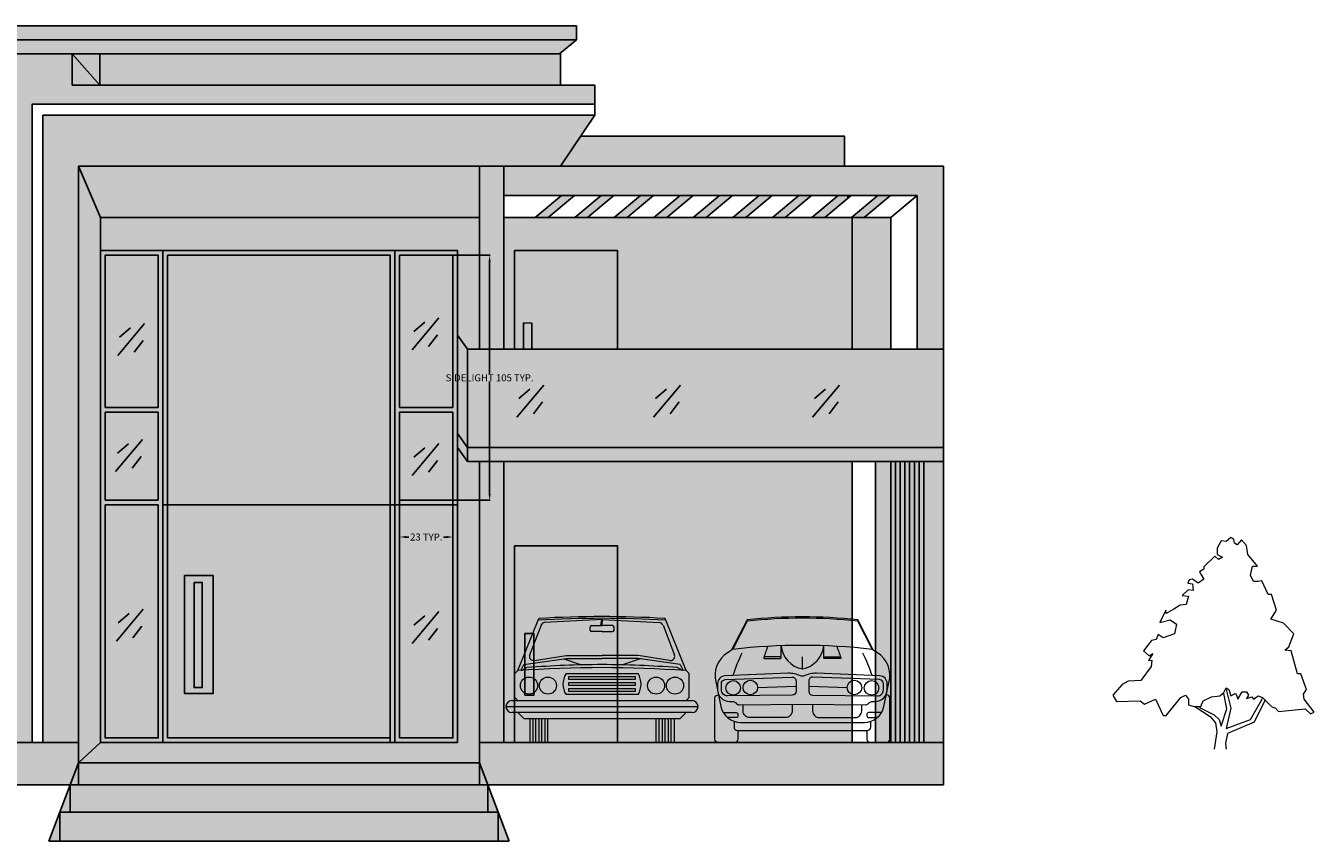
# Model space of a CAD drawing. Units: inches. Extents: x 13 to 1693, y -7 to 1519.
# Tile 7 of 10: x 292 to 842, y 1171 to 1519. Entities that reach past the tile are written whole.
import ezdxf

# ---------------------------------------------------------------- set-up
doc = ezdxf.new("R2010")
doc.units = ezdxf.units.IN
doc.header["$MEASUREMENT"] = 0
for name, color, linetype, lineweight in [('A-ANNO-DIMS', 2, 'Continuous', 18), ('A-ELEV', 7, 'Continuous', 25), ('A-ELEV-PATT', 8, 'Continuous', 13), ('A-EQPM', 8, 'Continuous', 18), ('TREE', 102, 'Continuous', 18)]:
    doc.layers.add(name, color=color, linetype=linetype, lineweight=lineweight)
doc.styles.get("Standard").update_dxf_attribs({"font": 'arial.ttf'})
doc.dimstyles.get("Standard").update_dxf_attribs({"dimtxt": 3, "dimasz": 2.68, "dimexe": 0.18, "dimexo": 0.0625, "dimgap": 0.09, "dimtad": 0, "dimtih": 1, "dimtoh": 1, "dimdec": 0, "dimzin": 0, "dimdsep": 46, "dimlunit": 3, "dimtxsty": 'Standard', "dimcen": 0.09, "dimadec": 0, "dimazin": 0, "dimtfac": 1, "dimtdec": 0, "dimtofl": 0, "dimtmove": 0, "dimatfit": 3, "dimfxl": 1, "dimtolj": 1, "dimtzin": 0, "dimarcsym": 0})

# ---------------------------------------------------------------- blocks, each defined once
blk = doc.blocks.new('*U27')
for p, q in [((-37.38, 32.04), (-28.11, 55.23)), ((-0.21, 54.74), (-0.67, 52.07)), ((0.21, 54.74), (-0.23, 52.08)), ((37.38, 32.04), (28.11, 55.23)), ((-36.05, 32.04), (-34.71, 34.71)), ((-34.71, 34.71), (-16.02, 37.38)), ((-16.94, 37.24), (-9.08, 34.62)), ((-16.02, 37.38), (0, 37.38)), ((16.02, 37.38), (0, 37.38)), ((16.93, 37.24), (9.08, 34.62)), ((34.71, 34.71), (16.02, 37.38)), ((34.71, 34.71), (36.05, 32.04)), ((-38.72, 30.71), (-37.38, 32.04)), ((-38.72, 20.03), (-38.72, 30.71)), ((-35.8, 32.16), (-33.38, 33.38)), ((-16.02, 30.71), (16.02, 30.71)), ((-14.69, 29.37), (14.69, 29.37)), ((-14.69, 28.04), (-14.69, 29.37)), ((14.69, 29.37), (14.69, 28.04)), ((35.8, 32.16), (33.38, 33.38)), ((38.72, 30.71), (37.38, 32.04)), ((38.72, 20.03), (38.72, 30.71)), ((14.69, 28.04), (-14.69, 28.04)), ((-14.69, 26.7), (14.69, 26.7)), ((-14.69, 25.37), (-14.69, 26.7)), ((14.69, 25.37), (-14.69, 25.37)), ((-14.69, 24.03), (14.69, 24.03)), ((-14.69, 22.7), (-14.69, 24.03)), ((14.69, 26.7), (14.69, 25.37)), ((14.69, 24.03), (14.69, 22.7)), ((-40.05, 18.69), (40.05, 18.69)), ((-37.38, 18.69), (-38.72, 20.03)), ((16.02, 21.36), (-16.02, 21.36)), ((14.69, 22.7), (-14.69, 22.7)), ((37.38, 18.69), (38.72, 20.03)), ((-42.72, 16.02), (42.72, 16.02)), ((40.05, 13.35), (-40.05, 13.35)), ((-37.38, 13.35), (-34.71, 10.68)), ((34.71, 10.68), (37.38, 13.35)), ((-34.71, 10.68), (34.71, 10.68)), ((-32.04, 10.68), (-32.04, 0)), ((-30.71, 10.68), (-30.71, 0)), ((-29.37, 0), (-29.37, 10.68)), ((-28.04, 10.68), (-28.04, 0)), ((-26.7, 0), (-26.7, 10.68)), ((-25.37, 10.68), (-25.37, 0)), ((-24.03, 0), (-24.03, 10.68)), ((24.03, 0), (24.03, 10.68)), ((25.37, 0), (25.37, 10.68)), ((26.7, 10.68), (26.7, 0)), ((28.04, 0), (28.04, 10.68)), ((29.37, 10.68), (29.37, 0)), ((30.71, 0), (30.71, 10.68)), ((32.04, 10.68), (32.04, 0)), ((-32.04, 0), (-24.03, 0)), ((32.04, 0), (24.03, 0))]:
    blk.add_line(p, q)
for points in [[(-27.12, 52.31), (-32.28, 38.89)], [(0, 54.74), (-25.63, 53.46)], [(-4.67, 52.07), (0, 52.07)], [(4.67, 52.07), (0, 52.07)], [(0.01, 54.74), (25.64, 53.45)], [(27.13, 52.3), (32.28, 38.88)], [(-5.34, 50.07), (-5.34, 51.4)], [(0, 49.4), (-4.67, 49.4)], [(0, 49.4), (4.67, 49.4)], [(5.34, 50.07), (5.34, 51.4)], [(-30.06, 36.56), (-16.02, 38.72), (0, 38.72)], [(30.06, 36.54), (16.02, 38.71), (0, 38.72)]]:
    blk.add_lwpolyline(points)
for centre in [(-32.47, 25.37), (-24.06, 25.37), (24.06, 25.37), (32.47, 25.37)]:
    blk.add_circle(centre, 3.8)
for centre, radius, start, end in [((0, -432), 487.32, 86.65721, 93.3419), ((0, -431.24), 487.32, 86.69396, 93.3033), ((-25.37, 51.59), 1.89, 97.4497, 154.9311), ((-4.67, 51.4), 0.668, 93.60832, 178.1081), ((4.67, 51.4), 0.668, 1.89193, 86.39168), ((25.37, 51.57), 1.89, 25.04208, 82.52346), ((-4.67, 50.07), 0.668, 184.4192, 266.4386), ((4.67, 50.07), 0.668, 273.5614, 355.5808), ((0.67, -399.87), 434.58, 90.08801, 94.49321), ((-30.43, 38.42), 1.89, 166.5724, 279.9572), ((-0.67, -399.87), 434.58, 85.50679, 89.91199), ((30.43, 38.41), 1.89, 260.016, 13.40079), ((0, -490.66), 524.03, 85.90918, 94.09081), ((-8.68, 26.03), 8.7, 147.5288, 212.4712), ((8.68, 26.03), 8.7, 327.5288, 32.47119), ((-40.05, 16.02), 2.67, 90, 270), ((40.05, 16.02), 2.67, 270, 90)]:
    blk.add_arc(centre, radius, start, end)
blk = doc.blocks.new('*U28')
for p, q in [((-9.51, 37.84), (-9.51, 43.25)), ((9.51, 37.84), (9.51, 43.25)), ((0, 32.82), (0, 38.19)), ((-19.91, 24.53), (-2.81, 25.14)), ((2.81, 25.14), (19.91, 24.53))]:
    blk.add_line(p, q)
for points in [[(-38.83, 28.63), (-36.22, 16.07, 0.355359), (-27.52, 9), (27.58, 9, 0.355331), (36.28, 16.07), (38.89, 28.63, 0.324597), (31.68, 40.93), (24.69, 54.68, 0.052145), (-24.63, 54.68), (-31.63, 40.93, 0.324597)], [(-24.58, 54.09), (-30.92, 41.61), (-30.92, 41.61, -0.059427), (30.98, 41.61), (24.64, 54.09, 0.05217)], [(-16.8, 37.38), (-9.88, 37.38, 0.414214), (-9.51, 37.75), (-9.51, 37.82, 0.414214), (-9.88, 38.19), (-16.8, 38.19, 0.414214), (-17.17, 37.82), (-17.17, 37.75, 0.414214)], [(16.8, 37.38), (9.88, 37.38, -0.414214), (9.51, 37.75), (9.51, 37.82, -0.414214), (9.88, 38.19), (16.8, 38.19, -0.414214), (17.17, 37.82), (17.17, 37.75, -0.414214)], [(-4.66, 29.17, -0.427329), (-2.81, 27.41), (-2.81, 22.88, -0.410558), (-4.56, 21.11), (-33.36, 20.8, -0.417878), (-36.04, 23.45), (-36.04, 26.26, -0.401219), (-34.35, 28.03)], [(4.66, 29.17, 0.427329), (2.81, 27.41), (2.81, 22.88, 0.410558), (4.56, 21.11), (33.36, 20.8, 0.417878), (36.04, 23.45), (36.04, 26.26, 0.401219), (34.35, 28.03)]]:
    blk.add_lwpolyline(points, format="xyb", close=True)
for points in [[(-6.29, 30.92), (-34.43, 29.71, 0.401219), (-37.73, 26.26), (-37.73, 23.63, 0.414214), (-32.43, 18.34), (-31.07, 18.34, -0.198912), (-29.82, 17.82), (-29.29, 17.29, 0.202778), (-28.01, 16.77), (0, 17.13), (28.01, 16.77, 0.202778), (29.29, 17.29), (29.82, 17.82, -0.198912), (31.07, 18.34), (32.43, 18.34, 0.414214), (37.73, 23.63), (37.73, 26.26, 0.401219), (34.43, 29.71), (6.29, 30.92)], [(6.29, 30.92, 0.105807), (0.87, 29.72, -0.131652), (-0.87, 29.72, 0.105807), (-6.29, 30.92)], [(-28.7, 5.37), (-28.7, 1.48, -0.414214), (-30.18, 0), (-37.41, 0, -0.414214), (-38.89, 1.48), (-38.89, 19.74, -0.414214), (-37.41, 21.22), (-37.29, 21.22)], [(28.7, 5.37), (28.7, 1.48, 0.414214), (30.18, 0), (37.41, 0, 0.414214), (38.89, 1.48), (38.89, 19.74, 0.414214), (37.41, 21.22), (37.35, 21.22)], [(-35.17, 13.37), (-29.44, 13.37, -0.414214), (-28.7, 12.63), (-28.7, 11.88, -0.414214), (-29.44, 11.14), (-33.31, 11.14)], [(-4.56, 17.07), (-4.56, 14.1, -0.414214), (-7.52, 11.14), (-23.43, 11.14, -0.414214), (-26.39, 14.1), (-26.39, 16.79)], [(4.56, 17.07), (4.56, 14.1, 0.414214), (7.52, 11.14), (23.43, 11.14, 0.414214), (26.39, 14.1), (26.39, 16.79)], [(35.17, 13.37), (29.44, 13.37, 0.414214), (28.7, 12.63), (28.7, 11.88, 0.414214), (29.44, 11.14), (33.31, 11.14)], [(-30.39, 9.47), (-30.39, 6.85, 0.414214), (-28.91, 5.37), (28.91, 5.37, 0.414214), (30.39, 6.85), (30.39, 9.47)]]:
    blk.add_lwpolyline(points, format="xyb")
for centre in [(-30.79, 24.36), (-23.15, 24.53), (23.15, 24.53), (30.79, 24.36)]:
    blk.add_circle(centre, 3.24)
for centre, radius, start, end in [((41.5, 19.77), 61.38, 157.83365, 162.90143), ((2.03, 44.22), 11.58, 184.78179, 259.90449), ((-2.03, 44.22), 11.58, 280.09551, 355.21821), ((-41.5, 19.77), 61.38, 17.09857, 22.16635), ((27.74, 11.77), 61.38, 152.82966, 162.90143), ((-27.69, 11.77), 61.38, 17.09857, 27.17034)]:
    blk.add_arc(centre, radius, start, end)
blk = doc.blocks.new('*U31')
for points in [[(22.0124, 137.721), (18.5475, 141.5624), (15.5282, 138.2446), (13.8028, 139.3505), (13.3714, 142.1153), (11.2148, 143.2214), (8.1954, 140.4564), (4.7447, 141.0094), (2.1567, 136.0326), (2.1567, 131.6088), (5.6074, 129.9499), (3.0193, 128.2909), (0.4313, 130.5029), (-6.9015, 123.3141), (-6.9015, 121.6552), (-9.9208, 119.9963), (-9.0581, 118.3373), (-6.9015, 115.0195), (-10.7835, 112.2546), (-14.6656, 115.0195), (-16.8222, 114.4665), (-17.6849, 112.2546), (-14.6656, 111.7016), (-14.2342, 107.2778), (-17.6065, 107.8307), (-21.5669, 103.9599), (-17.2536, 103.4069), (-18.9789, 97.8771), (-22.8609, 97.3241), (-27.1743, 94.5593), (-32.3504, 91.7944), (-32.7817, 94.0063), (-36.6638, 85.7116), (-29.7624, 87.3705), (-25.449, 84.6056), (-26.743, 77.9699), (-34.507, 75.205), (-37.9578, 77.4169), (-39.2518, 74.099), (-42.2711, 73.5461), (-44.8592, 70.2282), (-47.8786, 66.3574), (-43.9965, 63.0395), (-41.4085, 64.6985), (-44.3346, 59.8898), (-42.2089, 60.1377), (-42.5159, 55.7849), (-49.6039, 46.4502), (-58.2307, 45.8972), (-62.1127, 43.6853), (-68.5828, 36.4966), (-65.9947, 32.0727), (-50.0352, 32.6257), (-47.0159, 30.4138), (-39.6831, 33.7317), (-34.507, 22.6721), (-32.3504, 22.6721), (-22.4296, 34.8376), (-19.4102, 36.4966), (-17.2536, 33.7317), (-17.2536, 29.8608), (-13.8028, 28.7549), (-9.0581, 28.7549), (-7.3328, 32.6257), (-1.7254, 35.3906), (3.8821, 35.9436), (6.4701, 38.1555), (6.9014, 38.7085), (8.1954, 41.4734), (9.9208, 40.3674), (11.2148, 35.9436), (14.2341, 37.6025), (15.0968, 36.4966), (15.9595, 33.7317), (18.9789, 38.7085), (21.9982, 38.7085), (23.2922, 36.4966), (21.9982, 34.2847), (25.4489, 35.3906), (26.743, 33.7317), (29.7623, 35.9436), (32.7817, 34.8376), (38.8204, 28.7549), (41.4084, 27.6489), (43.5651, 25.437), (61.6813, 27.0959), (65.132, 23.7781), (67.7201, 24.884), (60.8186, 33.7317), (60.3873, 37.0495), (62.544, 40.3674), (58.662, 50.874), (56.5053, 50.874), (52.1919, 66.3574), (47.8785, 66.9103), (50.4665, 69.1222), (53.9172, 77.9699), (47.0158, 85.1586), (38.3891, 87.9235), (42.2711, 94.0063)], [(42.2711, 94.0063), (38.8204, 104.5129), (36.6637, 104.5129), (32.3503, 113.9135), (29.7623, 113.3605), (26.743, 113.3605), (24.5862, 117.7844), (25.8802, 123.8671), (29.331, 123.8671), (22.8609, 131.6088), (21.9982, 137.6916)], [(-9.9208, 28.2019), (0, 23.2251), (3.4507, 19.9072), (4.7447, 15.4834), (8.6267, 27.0959), (6.4701, 37.6025)], [(8.1954, 40.3674), (11.2148, 27.6489), (8.1954, 13.8245), (24.5862, 19.9072), (32.7817, 34.2847)], [(-12.9401, 28.7549), (-2.588, 22.1191), (0.8626, 17.6953), (1.7253, 11.6125), (0, 0)], [(34.5071, 33.1787), (27.1743, 18.2483), (9.0581, 10.5066), (7.7641, 3.8708), (8.1954, 0)]]:
    blk.add_lwpolyline(points)
blk = doc.blocks.new('ELEV-SIDELIGHT')
for p, q in [((22.68, 39.67), (0, 39.67)), ((22.68, 37.67), (0, 37.67)), ((0, 0), (22.68, 0))]:
    blk.add_line(p, q)
for points in [[(0, 39.67), (0, 104.56), (22.68, 104.56), (22.68, 39.67)], [(0, 0), (0, 37.67)], [(22.68, 37.67), (22.68, 0)]]:
    blk.add_lwpolyline(points)
blk = doc.blocks.new('*D66')
at = {"layer": 'A-ANNO-DIMS', "color": 0, "lineweight": -2, "transparency": 16777216}
for p, q in [((474.2, 1421.23), (490, 1421.23)), ((489.82, 1418.55), (489.82, 1370.59)), ((489.82, 1319.35), (489.82, 1367.31)), ((474.2, 1316.67), (490, 1316.67))]:
    blk.add_line(p, q, dxfattribs=at)
at = {"layer": 'A-ANNO-DIMS', "color": 0, "transparency": 16777216}
for points in [[(489.37, 1418.55), (490.27, 1418.55), (489.82, 1421.23)], [(489.37, 1319.35), (490.27, 1319.35), (489.82, 1316.67)]]:
    blk.add_solid(points, dxfattribs=at)
at = {"layer": 'Defpoints', "color": 0, "transparency": 16777216}
for p in [(474.14, 1421.23), (489.82, 1421.23), (474.14, 1316.67)]:
    blk.add_point(p, dxfattribs=at)
at = {"layer": 'A-ANNO-DIMS', "color": 0, "transparency": 16777216, "insert": (489.82, 1368.95), "char_height": 3, "attachment_point": 5}
blk.add_mtext('\\A1;SIDELIGHT 105 TYP.', dxfattribs=at)
blk = doc.blocks.new('*D67')
at = {"layer": 'A-ANNO-DIMS', "color": 0, "lineweight": -2, "transparency": 16777216}
for p, q in [((451.45, 1316.61), (451.45, 1300.81)), ((474.14, 1316.61), (474.14, 1300.81)), ((454.13, 1300.99), (455.38, 1300.99)), ((471.46, 1300.99), (470.21, 1300.99))]:
    blk.add_line(p, q, dxfattribs=at)
at = {"layer": 'A-ANNO-DIMS', "color": 0, "transparency": 16777216}
for points in [[(454.13, 1301.43), (454.13, 1300.54), (451.45, 1300.99)], [(471.46, 1301.43), (471.46, 1300.54), (474.14, 1300.99)]]:
    blk.add_solid(points, dxfattribs=at)
at = {"layer": 'Defpoints', "color": 0, "transparency": 16777216}
for p in [(451.45, 1316.67), (474.14, 1316.67), (474.14, 1300.99)]:
    blk.add_point(p, dxfattribs=at)
at = {"layer": 'A-ANNO-DIMS', "color": 0, "transparency": 16777216, "insert": (462.8, 1300.99), "char_height": 3, "attachment_point": 5}
blk.add_mtext('\\A1;23 TYP.', dxfattribs=at)

msp = doc.modelspace()

# ---------------------------------------------------------------- hatches: boundary and pattern name
at = {"layer": 'A-ELEV-PATT'}
h = msp.add_hatch(color=256, dxfattribs=at)
h.dxf.hatch_style = 1
h.paths.add_polyline_path([(526.9, 1519.22), (247.4, 1519.22), (247.4, 1513.22), (526.9, 1513.22)])
h = msp.add_hatch(color=256, dxfattribs=at)
h.dxf.hatch_style = 1
h.paths.add_polyline_path([(485.45, 1459.23), (314.45, 1459.23), (323.77, 1437.38), (485.45, 1437.38)])
h.paths.add_polyline_path([(323.77, 1437.38), (314.45, 1459.23), (314.45, 1204.63), (323.77, 1213.23), (323.77, 1423.23)])
h.paths.add_polyline_path([(526.9, 1513.22), (247.4, 1513.22), (267.64, 1507.23), (519.7, 1507.23)])
h = msp.add_hatch(color=256, dxfattribs=at)
h.dxf.hatch_style = 1
h.paths.add_polyline_path([(534.67, 1493.81), (311.73, 1493.81), (311.73, 1507.23), (169.4, 1507.23), (169.4, 1457.61), (259.19, 1457.61), (259.19, 1213.23), (294.63, 1213.23), (294.63, 1485.7), (299.21, 1485.7), (534.67, 1485.7)])
h.paths.add_polyline_path([(534.67, 1481.12), (299.21, 1481.12), (299.21, 1213.23), (314.45, 1213.23), (314.45, 1459.23), (520.13, 1459.23)], flags=17)
h.paths.add_polyline_path([(146.87, 1507.23), (116.45, 1507.23), (116.45, 1339.23), (116.45, 1213.23), (129.66, 1213.23), (129.66, 1457.61), (146.87, 1457.61)])
h.paths.add_polyline_path([(151, 1507.23), (148.74, 1507.23), (148.74, 1457.61), (151, 1457.61)])
h.paths.add_polyline_path([(155.13, 1507.23), (152.87, 1507.23), (152.87, 1457.61), (155.13, 1457.61)])
h.paths.add_polyline_path([(159.26, 1507.23), (157.01, 1507.23), (157.01, 1457.61), (159.26, 1457.61)])
h.paths.add_polyline_path([(163.39, 1507.23), (161.14, 1507.23), (161.14, 1457.61), (163.39, 1457.61)])
h.paths.add_polyline_path([(167.53, 1507.23), (165.27, 1507.23), (165.27, 1457.61), (167.53, 1457.61)])
h = msp.add_hatch(color=256, dxfattribs=at)
h.dxf.hatch_style = 1
h.paths.add_polyline_path([(323.53, 1507.23), (311.73, 1507.23), (323.53, 1493.81)], flags=17)
h.paths.add_polyline_path([(311.73, 1507.23), (311.73, 1493.81), (323.53, 1493.81)])
h = msp.add_hatch(color=256, dxfattribs=at)
h.dxf.hatch_style = 1
h.paths.add_polyline_path([(520.13, 1507.59), (519.7, 1507.23), (323.53, 1507.23), (323.53, 1493.81), (520.13, 1493.81)])
h = msp.add_hatch(color=256, dxfattribs=at)
h.dxf.hatch_style = 1
h.paths.add_polyline_path([(641.26, 1472.05), (528.65, 1472.05), (520.13, 1459.23), (641.26, 1459.23)])
h = msp.add_hatch(color=256, dxfattribs=at)
h.dxf.hatch_style = 1
h.paths.add_polyline_path([(495.89, 1459.23), (485.45, 1459.23), (485.45, 1381.23), (495.89, 1381.23)])
h.paths.add_polyline_path([(495.89, 1333.23), (485.45, 1333.23), (485.45, 1213.23), (495.89, 1213.23)])
h = msp.add_hatch(color=256, dxfattribs=at)
h.dxf.hatch_style = 1
h.paths.add_polyline_path([(683.45, 1459.23), (495.89, 1459.23), (495.89, 1446.73), (672.26, 1446.73), (672.26, 1381.23), (683.45, 1381.23)])
h.paths.add_polyline_path([(661.02, 1437.38), (644.49, 1437.38), (644.49, 1381.23), (661.02, 1381.23)], flags=17)
h = msp.add_hatch(color=256, dxfattribs=at)
h.dxf.hatch_style = 1
h.paths.add_polyline_path([(526.03, 1446.73), (520.54, 1446.73), (509.3, 1437.38), (514.79, 1437.38)])
h.paths.add_polyline_path([(542.89, 1446.73), (537.4, 1446.73), (526.16, 1437.38), (531.65, 1437.38)])
h.paths.add_polyline_path([(559.75, 1446.73), (554.25, 1446.73), (543.02, 1437.38), (548.51, 1437.38)])
h.paths.add_polyline_path([(576.6, 1446.73), (571.11, 1446.73), (559.87, 1437.38), (565.37, 1437.38)])
h.paths.add_polyline_path([(593.46, 1446.73), (587.97, 1446.73), (576.73, 1437.38), (582.22, 1437.38)])
h.paths.add_polyline_path([(610.32, 1446.73), (604.83, 1446.73), (593.59, 1437.38), (599.08, 1437.38)])
h.paths.add_polyline_path([(627.18, 1446.73), (621.68, 1446.73), (610.45, 1437.38), (615.94, 1437.38)])
h.paths.add_polyline_path([(642.63, 1445.56), (642.63, 1446.73), (638.54, 1446.73), (627.3, 1437.38), (632.8, 1437.38)])
h.paths.add_polyline_path([(660.89, 1446.73), (655.4, 1446.73), (644.16, 1437.38), (649.65, 1437.38)])
h = msp.add_hatch(color=256, dxfattribs=at)
h.dxf.hatch_style = 1
h.paths.add_polyline_path([(644.49, 1333.23), (495.89, 1333.23), (495.89, 1213.23), (500.45, 1213.23), (500.45, 1297.23), (544.41, 1297.23), (544.41, 1213.23), (644.49, 1213.23)])
h.paths.add_polyline_path([(644.49, 1437.38), (495.89, 1437.38), (495.89, 1381.23), (500.45, 1381.23), (500.45, 1423.23), (544.41, 1423.23), (544.41, 1381.23), (644.49, 1381.23)])
h.paths.add_polyline_path([(485.45, 1437.38), (323.77, 1437.38), (323.77, 1423.23), (350.45, 1423.23), (449.45, 1423.23), (476.14, 1423.23), (476.14, 1387.14), (480.46, 1381.23), (485.45, 1381.23)])
h.paths.add_polyline_path([(485.45, 1333.23), (480.46, 1333.23), (476.14, 1339.14), (476.14, 1213.23), (449.45, 1213.23), (323.77, 1213.23), (314.45, 1204.63), (485.45, 1204.63)])
at = {"layer": 'A-ELEV-PATT', "transparency": 33554592}
h = msp.add_hatch(color=256, dxfattribs=at)
h.dxf.hatch_style = 1
h.paths.add_polyline_path([(202.48, 1421.23), (175.34, 1421.23), (175.34, 1381.23), (175.34, 1354.34), (202.48, 1354.34)])
h.paths.add_polyline_path([(226.48, 1421.23), (211.36, 1421.23), (204.48, 1421.23), (204.48, 1354.34), (226.48, 1354.34)])
h.paths.add_polyline_path([(259.19, 1421.23), (228.48, 1421.23), (228.48, 1354.34), (259.19, 1354.34)])
h.paths.add_polyline_path([(259.19, 1316.67), (230.48, 1316.67), (230.48, 1251.23), (259.19, 1251.23)])
h.paths.add_polyline_path([(228.48, 1316.67), (206.48, 1316.67), (206.48, 1251.23), (228.48, 1251.23)])
h.paths.add_polyline_path([(204.48, 1316.67), (175.34, 1316.67), (175.34, 1297.23), (175.34, 1251.23), (204.48, 1251.23)])
h.paths.add_polyline_path([(480.46, 1381.23), (476.14, 1387.14), (476.14, 1345.14), (480.46, 1339.23)])
h.paths.add_polyline_path([(683.45, 1381.23), (480.46, 1381.23), (480.46, 1339.23), (683.45, 1339.23)])
h.paths.add_polyline_path([(348.45, 1421.23), (325.77, 1421.23), (325.77, 1356.34), (348.45, 1356.34)])
h.paths.add_polyline_path([(474.14, 1421.23), (451.45, 1421.23), (451.45, 1356.34), (474.14, 1356.34)])
h.paths.add_polyline_path([(474.14, 1354.34), (451.45, 1354.34), (451.45, 1316.67), (474.14, 1316.67)])
h.paths.add_polyline_path([(348.45, 1354.34), (325.77, 1354.34), (325.77, 1316.67), (348.45, 1316.67)])
h.paths.add_polyline_path([(348.45, 1314.67), (325.77, 1314.67), (325.77, 1215.23), (348.45, 1215.23)])
h.paths.add_polyline_path([(474.14, 1314.67), (451.45, 1314.67), (451.45, 1215.23), (474.14, 1215.23)])
at = {"layer": 'A-ELEV-PATT'}
h = msp.add_hatch(color=256, dxfattribs=at)
h.dxf.hatch_style = 1
h.paths.add_polyline_path([(350.45, 1423.23), (323.77, 1423.23), (323.77, 1213.23), (350.45, 1213.23)])
h.paths.add_polyline_path([(325.77, 1356.34), (325.77, 1421.23), (348.45, 1421.23), (348.45, 1356.34)], flags=16)
h.paths.add_polyline_path([(348.45, 1354.34), (348.45, 1316.67), (325.77, 1316.67), (325.77, 1354.34)], flags=16)
h.paths.add_polyline_path([(348.45, 1314.67), (348.45, 1215.23), (325.77, 1215.23), (325.77, 1314.67)], flags=16)
h = msp.add_hatch(color=256, dxfattribs=at)
h.dxf.hatch_style = 1
h.paths.add_polyline_path([(449.45, 1423.23), (350.45, 1423.23), (350.45, 1375.23), (350.45, 1314.67), (352.45, 1314.67), (352.45, 1375.23), (352.45, 1421.23), (447.45, 1421.23), (447.45, 1375.23), (447.45, 1314.67), (449.45, 1314.67), (449.45, 1375.23)])
h = msp.add_hatch(color=256, dxfattribs=at)
h.dxf.hatch_style = 1
h.paths.add_polyline_path([(447.45, 1375.23), (447.45, 1421.23), (352.45, 1421.23), (352.45, 1375.23), (352.45, 1314.67), (447.45, 1314.67)])
h = msp.add_hatch(color=256, dxfattribs=at)
h.dxf.hatch_style = 1
h.paths.add_polyline_path([(476.14, 1423.23), (449.45, 1423.23), (449.45, 1314.67), (476.14, 1314.67)])
h.paths.add_polyline_path([(474.14, 1356.34), (451.45, 1356.34), (451.45, 1421.23), (474.14, 1421.23)], flags=16)
h.paths.add_polyline_path([(474.14, 1354.34), (474.14, 1316.67), (451.45, 1316.67), (451.45, 1354.34)], flags=16)
h.paths.add_polyline_path([(476.14, 1314.67), (474.14, 1314.67), (474.14, 1215.23), (451.45, 1215.23), (451.45, 1314.67), (449.45, 1314.67), (449.45, 1213.23), (476.14, 1213.23)])
h = msp.add_hatch(color=256, dxfattribs=at)
h.dxf.hatch_style = 1
h.paths.add_polyline_path([(544.41, 1423.23), (500.45, 1423.23), (500.45, 1381.23), (504.32, 1381.23), (504.32, 1392.37), (507.79, 1392.31), (507.79, 1381.23), (544.41, 1381.23)])
h = msp.add_hatch(color=256, dxfattribs=at)
h.dxf.hatch_style = 1
h.paths.add_polyline_path([(507.79, 1392.31), (504.32, 1392.37), (504.32, 1381.3), (507.79, 1381.23)])
h = msp.add_hatch(color=256, dxfattribs=at)
h.dxf.hatch_style = 1
h.paths.add_polyline_path([(683.45, 1339.23), (480.46, 1339.23), (480.46, 1333.23), (683.45, 1333.23)])
h.paths.add_polyline_path([(476.14, 1345.14), (476.14, 1339.14), (480.46, 1333.23), (480.46, 1339.23)])
h = msp.add_hatch(color=256, dxfattribs=at)
h.dxf.hatch_style = 1
h.paths.add_polyline_path([(661.02, 1333.23), (654.43, 1333.23), (654.43, 1213.23), (661.02, 1213.23)])
h = msp.add_hatch(color=256, dxfattribs=at)
h.dxf.hatch_style = 1
h.paths.add_polyline_path([(663.02, 1333.23), (661.02, 1333.23), (661.02, 1213.23), (663.02, 1213.23)])
h.paths.add_polyline_path([(667.02, 1333.23), (665.02, 1333.23), (665.02, 1213.23), (667.02, 1213.23)])
h.paths.add_polyline_path([(671.02, 1333.23), (669.02, 1333.23), (669.02, 1213.23), (671.02, 1213.23)])
h.paths.add_polyline_path([(665.02, 1333.23), (663.02, 1333.23), (663.02, 1213.23), (665.02, 1213.23)])
h = msp.add_hatch(color=256, dxfattribs=at)
h.dxf.hatch_style = 1
h.paths.add_polyline_path([(665.02, 1333.23), (663.02, 1333.23), (663.02, 1213.23)])
h = msp.add_hatch(color=256, dxfattribs=at)
h.dxf.hatch_style = 1
h.paths.add_polyline_path([(673.02, 1333.23), (671.02, 1333.23), (671.02, 1213.23), (673.02, 1213.23)])
h.paths.add_polyline_path([(675.02, 1333.23), (673.02, 1333.23), (673.02, 1213.23), (675.02, 1213.23)])
h.paths.add_polyline_path([(669.02, 1333.23), (667.02, 1333.23), (667.02, 1213.23), (669.02, 1213.23)])
h = msp.add_hatch(color=256, dxfattribs=at)
h.dxf.hatch_style = 1
h.paths.add_polyline_path([(683.45, 1333.23), (675.02, 1333.23), (675.02, 1213.23), (683.45, 1213.23)])
h = msp.add_hatch(color=256, dxfattribs=at)
h.dxf.hatch_style = 1
h.paths.add_polyline_path([(352.45, 1314.67), (350.45, 1314.67), (350.45, 1297.23), (350.45, 1213.23), (399.95, 1213.23), (447.45, 1213.23), (447.45, 1215.23), (399.95, 1215.23), (352.45, 1215.23), (352.45, 1297.23)])
h.paths.add_polyline_path([(449.45, 1297.23), (449.45, 1314.67), (447.45, 1314.67), (447.45, 1213.23), (449.45, 1213.23)])
h = msp.add_hatch(color=256, dxfattribs=at)
h.dxf.hatch_style = 1
h.paths.add_polyline_path([(352.45, 1314.67), (352.45, 1297.23), (352.45, 1215.23), (399.95, 1215.23), (447.45, 1215.23), (447.45, 1297.23), (447.45, 1314.67)])
h.paths.add_polyline_path([(371.9, 1284.52), (371.9, 1234.22), (359.62, 1234.22), (359.62, 1284.52)], flags=16)
h = msp.add_hatch(color=256, dxfattribs=at)
h.dxf.hatch_style = 1
h.paths.add_polyline_path([(544.41, 1297.23), (500.45, 1297.23), (500.45, 1213.23), (544.41, 1213.23)])
h.paths.add_polyline_path([(508.74, 1259.76), (508.74, 1233.51), (504.9, 1233.51), (504.9, 1259.76)], flags=16)
h = msp.add_hatch(color=256, dxfattribs=at)
h.dxf.hatch_style = 1
h.paths.add_polyline_path([(359.62, 1284.52), (359.62, 1234.22), (371.9, 1234.22), (371.9, 1284.52)])
h = msp.add_hatch(color=256, dxfattribs=at)
h.dxf.hatch_style = 1
h.paths.add_polyline_path([(367.22, 1281.62), (363.72, 1281.62), (363.72, 1236.7), (367.22, 1236.7)])
h = msp.add_hatch(color=256, dxfattribs=at)
h.dxf.hatch_style = 1
h.paths.add_polyline_path([(508.74, 1259.76), (504.9, 1259.76), (504.9, 1233.51), (508.74, 1233.51)])
h = msp.add_hatch(dxfattribs=at)
h.set_pattern_fill('AR-CONC', color=256)
h.set_pattern_definition([(50, (-1203.873, -530.7854), (7.172602, -0.627521), [0.75, -8.25]), (355, (-1203.873, -530.785), (-1.387513, 7.521921), [0.6, -6.6]), (100.45144, (-1203.2755, -530.8376), (5.785088, 6.8944), [0.637402, -7.011421]), (46.1842, (-1203.873, -528.785), (10.672413, -1.655193), [1.125, -12.375]), (96.63564, (-1202.984, -528.923), (9.34662, 9.741186), [0.956103, -10.517138]), (351.18416, (-1203.873, -528.785), (9.34662, 9.741186), [0.9, -9.9]), (21, (-1202.873, -529.2854), (5.96907, -4.026189), [0.75, -8.25]), (326, (-1202.873, -529.285), (2.433153, 7.2515), [0.6, -6.6]), (71.45144, (-1202.376, -529.621), (8.402224, 3.225312), [0.637402, -7.011421]), (37.5, (-1203.8732, -530.7854), (0.1215986, 3.3289385), [0, -6.52, 0, -6.7, 0, -6.625]), (7.5, (-1203.8732, -530.7854), (2.6306954, 3.944117), [0, -3.82, 0, -6.37, 0, -2.525]), (327.5, (-1206.1032, -530.7854), (5.3382244, -0.2255487), [0, -2.5, 0, -7.8, 0, -10.35]), (317.5, (-1207.103, -530.7854), (5.831862, 1.00105), [0, -3.25, 0, -5.18, 0, -7.35])])
h.paths.add_polyline_path([(314.45, 1213.23), (116.45, 1213.23), (116.45, 1195.23), (310.89, 1195.23), (314.45, 1204.63)])
h.paths.add_polyline_path([(683.45, 1213.23), (485.45, 1213.23), (485.45, 1204.63), (489.01, 1195.23), (683.45, 1195.23)])
h = msp.add_hatch(color=256, dxfattribs=at)
h.dxf.hatch_style = 1
h.paths.add_polyline_path([(485.45, 1204.63), (314.45, 1204.63), (314.45, 1195.23), (485.45, 1195.23)])
h.paths.add_polyline_path([(489.01, 1195.23), (310.89, 1195.23), (310.89, 1183.6), (489.01, 1183.6)])
h.paths.add_polyline_path([(493.42, 1183.6), (306.49, 1183.6), (306.49, 1171.13), (493.42, 1171.13)])
h.paths.add_polyline_path([(314.45, 1204.63), (310.89, 1195.23), (314.45, 1195.23)])
h.paths.add_polyline_path([(310.89, 1195.23), (306.49, 1183.6), (310.89, 1183.6)])
h.paths.add_polyline_path([(306.49, 1183.6), (301.76, 1171.13), (306.49, 1171.13)])
h.paths.add_polyline_path([(493.42, 1183.6), (493.42, 1171.13), (498.14, 1171.13)])
h.paths.add_polyline_path([(489.01, 1195.23), (489.01, 1183.6), (493.42, 1183.6)])
h.paths.add_polyline_path([(485.45, 1204.63), (485.45, 1195.23), (489.01, 1195.23)])

# ---------------------------------------------------------------- linework, layer by layer
at = {"layer": 'A-ELEV'}
for p, q in [((247.4, 1519.22), (526.9, 1519.22)), ((526.9, 1519.22), (526.9, 1513.22)), ((247.4, 1513.22), (526.9, 1513.22)), ((526.9, 1513.22), (519.7, 1507.23)), ((116.45, 1507.23), (519.7, 1507.23)), ((311.73, 1507.23), (311.73, 1493.81)), ((311.73, 1507.23), (323.53, 1493.81)), ((323.53, 1507.23), (323.53, 1493.81)), ((520.13, 1507.23), (520.13, 1493.81)), ((311.73, 1493.81), (534.67, 1493.81)), ((534.67, 1493.81), (534.67, 1485.7)), ((534.67, 1481.12), (520.13, 1459.23)), ((314.45, 1204.63), (314.45, 1459.23)), ((314.45, 1459.23), (323.77, 1437.38)), ((485.45, 1381.23), (485.45, 1459.23)), ((495.89, 1459.23), (495.89, 1381.23)), ((683.45, 1459.23), (683.45, 1381.23)), ((495.89, 1446.73), (495.89, 1446.73)), ((495.89, 1446.73), (672.26, 1446.73)), ((520.54, 1446.73), (509.3, 1437.38)), ((526.03, 1446.73), (514.79, 1437.38)), ((537.4, 1446.73), (526.16, 1437.38)), ((542.89, 1446.73), (531.65, 1437.38)), ((554.25, 1446.73), (543.02, 1437.38)), ((559.75, 1446.73), (548.51, 1437.38)), ((571.11, 1446.73), (559.87, 1437.38)), ((576.6, 1446.73), (565.37, 1437.38)), ((587.97, 1446.73), (576.73, 1437.38)), ((593.46, 1446.73), (582.22, 1437.38)), ((604.83, 1446.73), (593.59, 1437.38)), ((610.32, 1446.73), (599.08, 1437.38)), ((621.68, 1446.73), (610.45, 1437.38)), ((627.18, 1446.73), (615.94, 1437.38)), ((638.54, 1446.73), (627.3, 1437.38)), ((644.03, 1446.73), (632.8, 1437.38)), ((642.63, 1446.73), (642.63, 1445.56)), ((655.4, 1446.73), (644.16, 1437.38)), ((660.89, 1446.73), (649.65, 1437.38)), ((672.26, 1446.73), (661.02, 1437.38)), ((672.26, 1446.73), (672.26, 1381.23)), ((323.77, 1423.23), (323.77, 1437.38)), ((485.45, 1437.38), (323.77, 1437.38)), ((661.02, 1437.38), (495.89, 1437.38)), ((644.49, 1437.38), (644.49, 1381.23)), ((661.02, 1437.38), (661.02, 1381.23)), ((342.65, 1392.15), (331.16, 1378.5)), ((468.21, 1394.53), (456.72, 1380.88)), ((462.23, 1392.71), (457.54, 1388.73)), ((336.67, 1390.33), (331.98, 1386.34)), ((467.62, 1387.32), (463.76, 1382.29)), ((480.46, 1381.23), (476.14, 1387.14)), ((342.06, 1384.94), (338.19, 1379.9)), ((480.46, 1381.23), (683.45, 1381.23)), ((480.46, 1381.23), (480.46, 1333.23)), ((683.45, 1381.23), (683.45, 1213.23)), ((683.45, 1381.23), (683.45, 1339.23)), ((350.45, 1375.23), (350.45, 1297.23)), ((352.45, 1375.23), (352.45, 1297.23)), ((447.45, 1375.23), (447.45, 1213.23)), ((449.45, 1375.23), (449.45, 1213.23)), ((512.98, 1365.86), (501.49, 1352.2)), ((507, 1364.04), (502.31, 1360.05)), ((571.26, 1365.86), (559.77, 1352.2)), ((565.28, 1364.04), (560.59, 1360.05)), ((639.13, 1365.86), (627.64, 1352.2)), ((633.16, 1364.04), (628.47, 1360.05)), ((512.39, 1358.65), (508.52, 1353.61)), ((570.68, 1358.65), (566.81, 1353.61)), ((638.55, 1358.65), (634.68, 1353.61)), ((341.74, 1342.61), (330.26, 1328.96)), ((480.46, 1339.23), (476.14, 1345.14)), ((335.77, 1340.79), (331.08, 1336.81)), ((468.21, 1340.85), (456.72, 1327.2)), ((462.23, 1339.03), (457.54, 1335.05)), ((480.46, 1333.23), (476.14, 1339.14)), ((480.46, 1339.23), (683.45, 1339.23)), ((683.45, 1339.23), (683.45, 1333.23)), ((341.16, 1335.4), (337.29, 1330.37)), ((467.62, 1333.64), (463.76, 1328.6)), ((683.45, 1333.23), (480.46, 1333.23)), ((485.45, 1204.63), (485.45, 1333.23)), ((495.89, 1333.23), (495.89, 1213.23)), ((644.49, 1213.23), (644.49, 1333.23)), ((654.43, 1333.23), (654.43, 1213.23)), ((661.02, 1213.23), (661.02, 1333.23)), ((661.02, 1213.23), (661.02, 1333.23)), ((663.02, 1213.23), (663.02, 1333.23)), ((665.02, 1213.23), (665.02, 1333.23)), ((667.02, 1213.23), (667.02, 1333.23)), ((669.02, 1213.23), (669.02, 1333.23)), ((669.02, 1213.23), (669.02, 1333.23)), ((669.02, 1213.23), (669.02, 1333.23)), ((671.02, 1213.23), (671.02, 1333.23)), ((673.02, 1213.23), (673.02, 1333.23)), ((675.02, 1213.23), (675.02, 1333.23)), ((325.77, 1314.67), (348.45, 1314.67)), ((350.45, 1314.67), (476.14, 1314.67)), ((342.09, 1270.15), (330.6, 1256.5)), ((336.11, 1268.33), (331.42, 1264.35)), ((468.21, 1269.19), (456.72, 1255.54)), ((462.23, 1267.37), (457.54, 1263.39)), ((341.51, 1262.94), (337.64, 1257.91)), ((467.62, 1261.98), (463.76, 1256.94)), ((323.77, 1213.23), (314.45, 1204.63)), ((314.45, 1204.63), (301.76, 1171.13)), ((314.45, 1204.63), (485.45, 1204.63)), ((314.45, 1204.63), (314.45, 1195.23)), ((485.45, 1204.63), (498.14, 1171.13)), ((485.45, 1204.63), (485.45, 1195.23)), ((310.89, 1195.23), (310.89, 1183.6)), ((489.01, 1195.23), (489.01, 1183.6)), ((306.49, 1183.6), (493.42, 1183.6)), ((306.49, 1183.6), (306.49, 1171.13)), ((493.42, 1183.6), (493.42, 1171.13)), ((301.76, 1171.13), (498.14, 1171.13))]:
    msp.add_line(p, q, dxfattribs=at)
for points in [[(299.21, 1481.12), (299.21, 1213.23), (294.63, 1213.23), (294.63, 1485.7), (299.21, 1485.7)], [(294.63, 1481.12), (294.63, 1485.7), (534.67, 1485.7), (534.67, 1481.12), (299.21, 1481.12)], [(528.65, 1472.05), (641.26, 1472.05), (641.26, 1459.23), (527.63, 1459.23)], [(683.45, 1459.23), (314.45, 1459.23)], [(449.45, 1375.23), (449.45, 1423.23), (350.45, 1423.23), (350.45, 1375.23)], [(447.45, 1375.23), (447.45, 1421.23), (352.45, 1421.23), (352.45, 1375.23)], [(500.45, 1381.23), (500.45, 1423.23), (544.41, 1423.23), (544.41, 1381.23)], [(348.45, 1314.67), (348.45, 1215.23), (325.77, 1215.23), (325.77, 1314.67)], [(474.14, 1314.67), (474.14, 1215.23), (451.45, 1215.23), (451.45, 1314.67)], [(399.95, 1213.23), (350.45, 1213.23), (350.45, 1297.23)], [(399.95, 1215.23), (352.45, 1215.23), (352.45, 1297.23)], [(449.45, 1297.23), (449.45, 1213.23), (399.95, 1213.23)], [(447.45, 1297.23), (447.45, 1215.23), (399.95, 1215.23)], [(485.45, 1213.23), (683.45, 1213.23), (683.45, 1195.23), (116.45, 1195.23), (116.45, 1213.23), (314.45, 1213.23)], [(323.77, 1213.23), (476.14, 1213.23)]]:
    msp.add_lwpolyline(points, dxfattribs=at)
for points in [[(350.45, 1213.23), (323.77, 1213.23), (323.77, 1423.23), (350.45, 1423.23)], [(476.14, 1213.23), (449.45, 1213.23), (449.45, 1423.23), (476.14, 1423.23)], [(504.32, 1392.37), (507.79, 1392.31), (507.79, 1381.23), (504.32, 1381.3)], [(544.41, 1213.23), (500.45, 1213.23), (500.45, 1297.23), (544.41, 1297.23)], [(359.62, 1284.52), (371.9, 1284.52), (371.9, 1234.22), (359.62, 1234.22)], [(363.72, 1281.62), (367.22, 1281.62), (367.22, 1236.7), (363.72, 1236.7)], [(504.9, 1259.76), (508.74, 1259.76), (508.74, 1233.51), (504.9, 1233.51)]]:
    msp.add_lwpolyline(points, close=True, dxfattribs=at)

# ---------------------------------------------------------------- block references
for p in [(325.77, 1316.67), (451.45, 1316.67)]:
    msp.add_blockref('ELEV-SIDELIGHT', p, dxfattribs=at)
at = {"layer": 'A-EQPM', "xscale": 0.9589998270527551, "yscale": 0.9589998270527551, "zscale": 0.9589998270527551}
for name, p in [('*U27', (537.78, 1213.23)), ('*U28', (623.26, 1213.23))]:
    msp.add_blockref(name, p, dxfattribs=at)
at = {"layer": 'TREE', "xscale": 0.6306016840312548, "yscale": 0.6306016840312548, "zscale": 0.6306016840312548}
msp.add_blockref('*U31', (798.91, 1210.5), dxfattribs=at)

# ---------------------------------------------------------------- dimensions: what is measured, and where the dimension line sits
at = {"layer": 'A-ANNO-DIMS'}
dim = msp.add_linear_dim(base=(489.82, 1421.23), p1=(474.14, 1316.67), p2=(474.14, 1421.23), angle=90, text='SIDELIGHT <> TYP.', dimstyle='Standard', override={"dimdec": 0, "dimlfac": 1, "dimrnd": 0, "dimzin": 0, "dimdsep": 46, "dimlunit": 2}, dxfattribs=at)
dim.commit()
dim.dimension.update_dxf_attribs({"geometry": '*D66', "text_midpoint": (489.82, 1368.95)})
dim = msp.add_linear_dim(base=(474.14, 1300.99), p1=(451.45, 1316.67), p2=(474.14, 1316.67), text='<> TYP.', dimstyle='Standard', override={"dimdec": 0, "dimlfac": 1, "dimrnd": 0, "dimzin": 0, "dimdsep": 46, "dimlunit": 2}, dxfattribs=at)
dim.commit()
dim.dimension.update_dxf_attribs({"geometry": '*D67', "text_midpoint": (462.8, 1300.99)})

doc.saveas('drawing.dxf')
